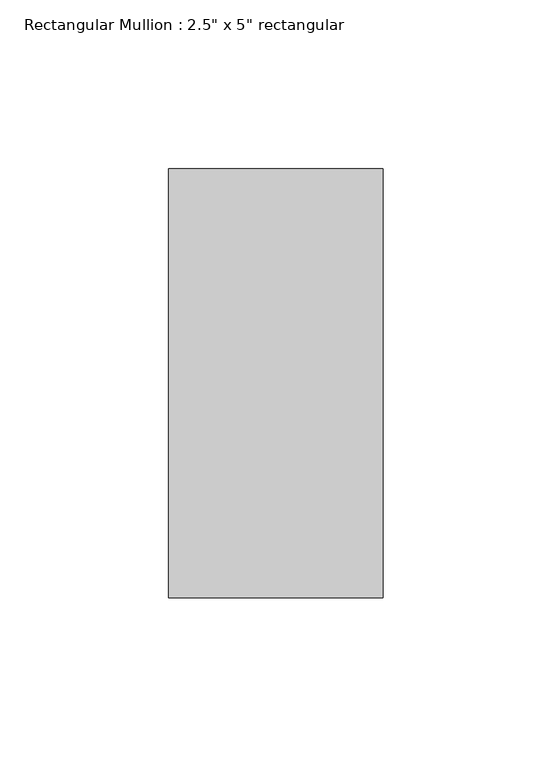
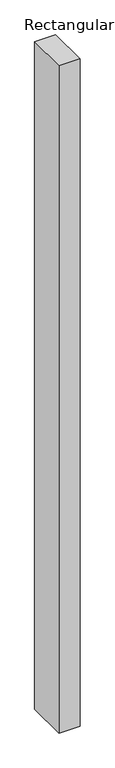
"""IFC4 building model written with IfcOpenShell, lengths in millimetres: member geometry."""

from ifc_helpers import new_model, si_unit, frame, origin, place, context, project, spatial, polyline, outline, extrude, source, transform, mapped, element, save


def member_3374d9b6(model_context):
    return source(origin(), model_context, "Body", "SweptSolid", [
        extrude(outline(polyline([(0.0, 63.5), (0.0, -63.5), (-63.5, -63.5), (-63.5, 63.5), (0.0, 63.5)])), frame((0.0, 0.0, -2133.6), z_axis=(0.0, 0.0, 1.0), x_axis=(1.0, 0.0, 0.0)), (0.0, 0.0, 1.0), 2133.6),
    ])


if __name__ == "__main__":
    model = new_model("IFC4")
    model_context = context("Model", 3, world=origin())
    ifc_project = project(units=[si_unit("LENGTHUNIT", "METRE", prefix="MILLI")], contexts=[model_context])
    site = spatial("IfcSite", under=ifc_project)
    building = spatial("IfcBuilding", under=site)
    placement = place(None, origin())
    member_shape = member_3374d9b6(model_context)
    element("IfcMember", 1, ObjectType="Rectangular Mullion : 2.5\" x 5\" rectangular", at=placement, inside=building, context=model_context, shape_type="MappedRepresentation", body=[
        mapped(member_shape, transform((0.0, 0.0, 0.0), x_axis=(1.0, 0.0, 0.0), y_axis=(0.0, 1.0, 0.0), z_axis=(0.0, 0.0, 1.0))),
    ])
    save(model, "model.ifc")

# Revit data of these elements
# Type "Rectangular Mullion : 2.5\" x 5\" rectangular"
#   built-in parameter 1007304 = 0.416667 (stored number, unit not read)
#   built-in parameter 1007301 = 0.104167 (stored number, unit not read)
#   built-in parameter 1007300 = 0.104167 (stored number, unit not read)
